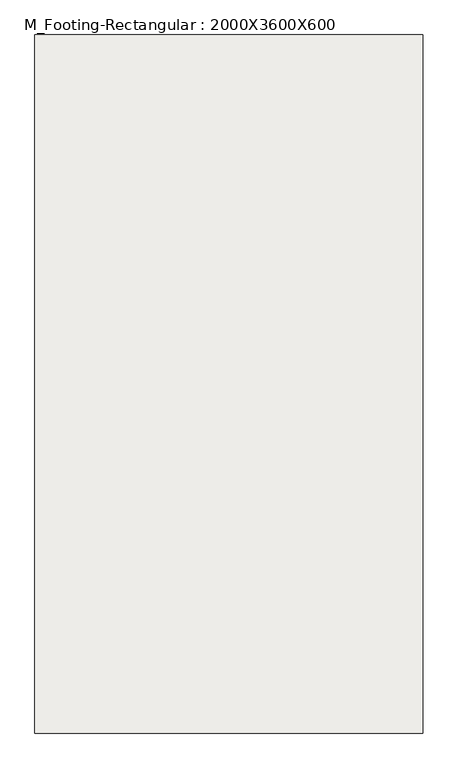
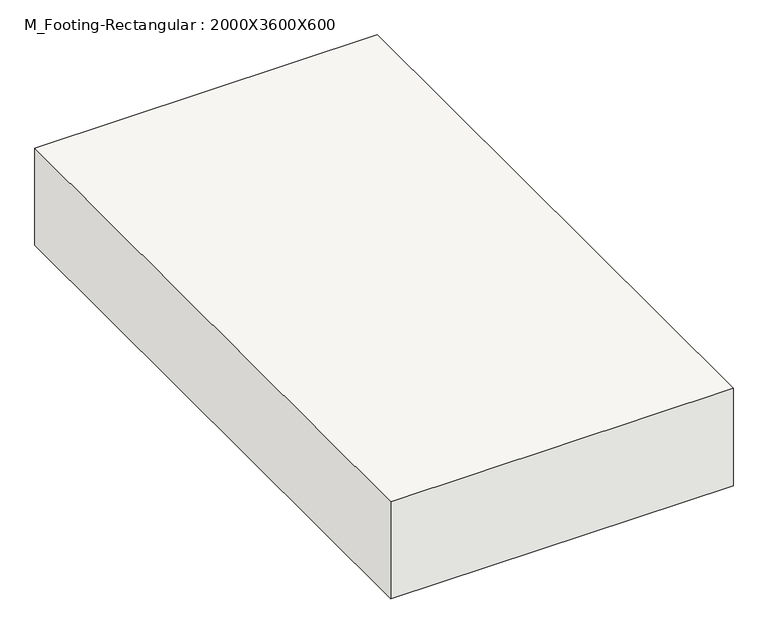
"""IFC4 building model written with IfcOpenShell, lengths in millimetres: slab geometry, M_Footing-Rectangular : 2000X3600X600."""

from ifc_helpers import new_model, si_unit, frame, origin, place, context, project, spatial, polyline, outline, extrude, source, transform, mapped, element, save


def m_footing_rectangular_2000x3600x600_ead935d4(model_context):
    return source(origin(), model_context, "Body", "SweptSolid", [
        extrude(outline(polyline([(1000.0, 1800.0), (1000.0, -1800.0), (-1000.0, -1800.0), (-1000.0, 1800.0), (1000.0, 1800.0)])), frame((0.0, 0.0, -600.0), z_axis=(0.0, 0.0, 1.0), x_axis=(1.0, 0.0, 0.0)), (0.0, 0.0, 1.0), 600.0),
    ])


if __name__ == "__main__":
    model = new_model("IFC4")
    model_context = context("Model", 3, world=origin())
    ifc_project = project(units=[si_unit("LENGTHUNIT", "METRE", prefix="MILLI")], contexts=[model_context])
    site = spatial("IfcSite", under=ifc_project)
    building = spatial("IfcBuilding", under=site)
    placement = place(None, origin())
    m_footing_rectangular_2000x3600x600_shape = m_footing_rectangular_2000x3600x600_ead935d4(model_context)
    element("IfcSlab", 1, ObjectType="M_Footing-Rectangular : 2000X3600X600", at=placement, inside=building, context=model_context, shape_type="MappedRepresentation", body=[
        mapped(m_footing_rectangular_2000x3600x600_shape, transform((0.0, 0.0, 0.0), x_axis=(1.0, 0.0, 0.0), y_axis=(0.0, 1.0, 0.0), z_axis=(0.0, 0.0, 1.0))),
    ])
    save(model, "model.ifc")

# Revit data of these elements
# Type "M_Footing-Rectangular : 2000X3600X600"
#   Width = 2000 mm
#   Length = 3600 mm
#   Foundation Thickness = 600 mm
#   Structural Material [instance default] = Concrete, Cast-in-Place gray
#   Assembly Code = ""
# Element 1 (IfcSlab, "M_Footing-Rectangular : 2000X3600X600")
#   Structural Material = Concrete, Cast In Situ
#   Materials on its faces: "Concrete, Cast In Situ"
# Materials
#   "Concrete, Cast-in-Place gray": class "Concrete", colour RGB 192 192 192, transparency 0, Description = "Cast-in-place concrete", Cost = 0
#   "Concrete, Cast In Situ": class "Concrete", colour RGB 192 192 192, transparency 0, Description = "physical material", Cost = 0
